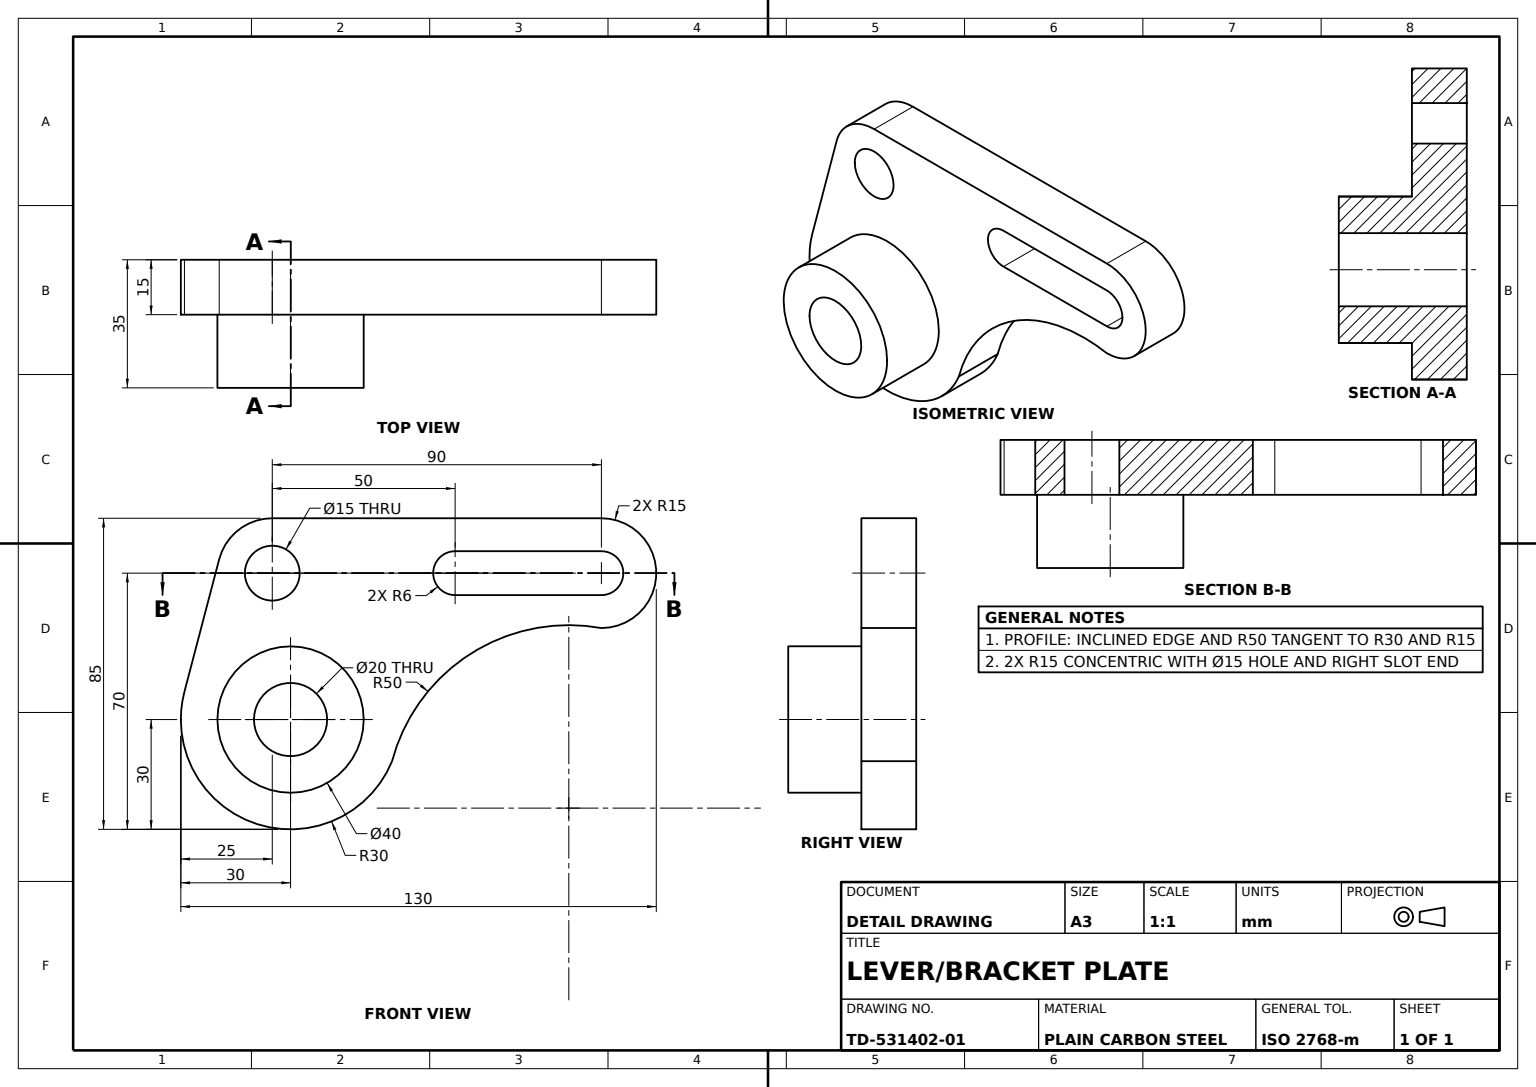
SolidWorks part; units mm, degrees
material "Plain Carbon Steel"
ref_plane "Front Plane" through (0, 0, 0) normal (0, 0, 1) x (1, 0, 0)
ref_plane "Top Plane" through (0, 0, 0) normal (0, 1, 0) x (1, 0, 0)
ref_plane "Right Plane" through (0, 0, 0) normal (1, 0, 0) x (0, 0, -1)
sketch "Lever Plate Profile" plane through (0, 0, 0) normal (0, 0, 1) x (1, 0, 0)
  line L0 (15, 0) -> (105, 0)
  line L4 (-9.0153, -47.3769) -> (0.4923, -11.1885)
  arc A0 (15, 0) -> (0.4923, -11.1885) centre (15, -15) ccw
  arc A2 (105, -30) -> (105, 0) centre (105, -15) ccw
  arc A3 (-9.0153, -47.3769) -> (47.7526, -66.3928) centre (20, -55) ccw
  arc A4 (47.7526, -66.3928) -> (105, -30) centre (96.0848, -79.1988) cw
  point P6 (0, 0)
  dimension "D1" = 15
  dimension "D2" = 30
  dimension "D3" = 90
  dimension "D4" = 60
  dimension "D5" = 30
  dimension "D6" = 50
  dimension "D7" = 9.0153
  dimension "D8" = 9.5077
  dimension "D9" = 24.0153
  dimension "D10" = 56.7679
extrude "Lever Plate" add sketch "Lever Plate Profile" along normal blind 15
sketch "Hub Profile" plane through (0, 0, 15) normal (0, 0, 1) x (1, 0, 0)
  circle A0 centre (20, -55) radius 20
  dimension "D1" = 40
  dimension "D2" = 40
extrude "Hub Ø40" add sketch "Hub Profile" along normal blind 20
sketch "Hub Bore Profile" plane through (0, 0, 35) normal (0, 0, 1) x (1, 0, 0)
  circle A0 centre (20, -55) radius 10
  dimension "D1" = 20
  dimension "D2" = 20
extrude "Hub Bore Ø20" cut sketch "Hub Bore Profile" against normal blind 35
sketch "Hole Profile" plane through (0, 0, 15) normal (0, 0, 1) x (1, 0, 0)
  circle A0 centre (15, -15) radius 7.5
  dimension "D1" = 15
  dimension "D2" = 15
extrude "Hole Ø15" cut sketch "Hole Profile" against normal blind 15
sketch "Slot Profile" plane through (0, 0, 15) normal (0, 0, 1) x (1, 0, 0)
  line L1 (65, -9) -> (105, -9)
  line L3 (105, -21) -> (65, -21)
  arc A0 (105, -21) -> (105, -9) centre (105, -15) ccw
  arc A1 (65, -9) -> (65, -21) centre (65, -15) ccw
  dimension "D1" = 12
  dimension "D2" = 12
  dimension "D3" = 6
  dimension "D4" = 50
extrude "Slot 12mm" cut sketch "Slot Profile" against normal blind 15
